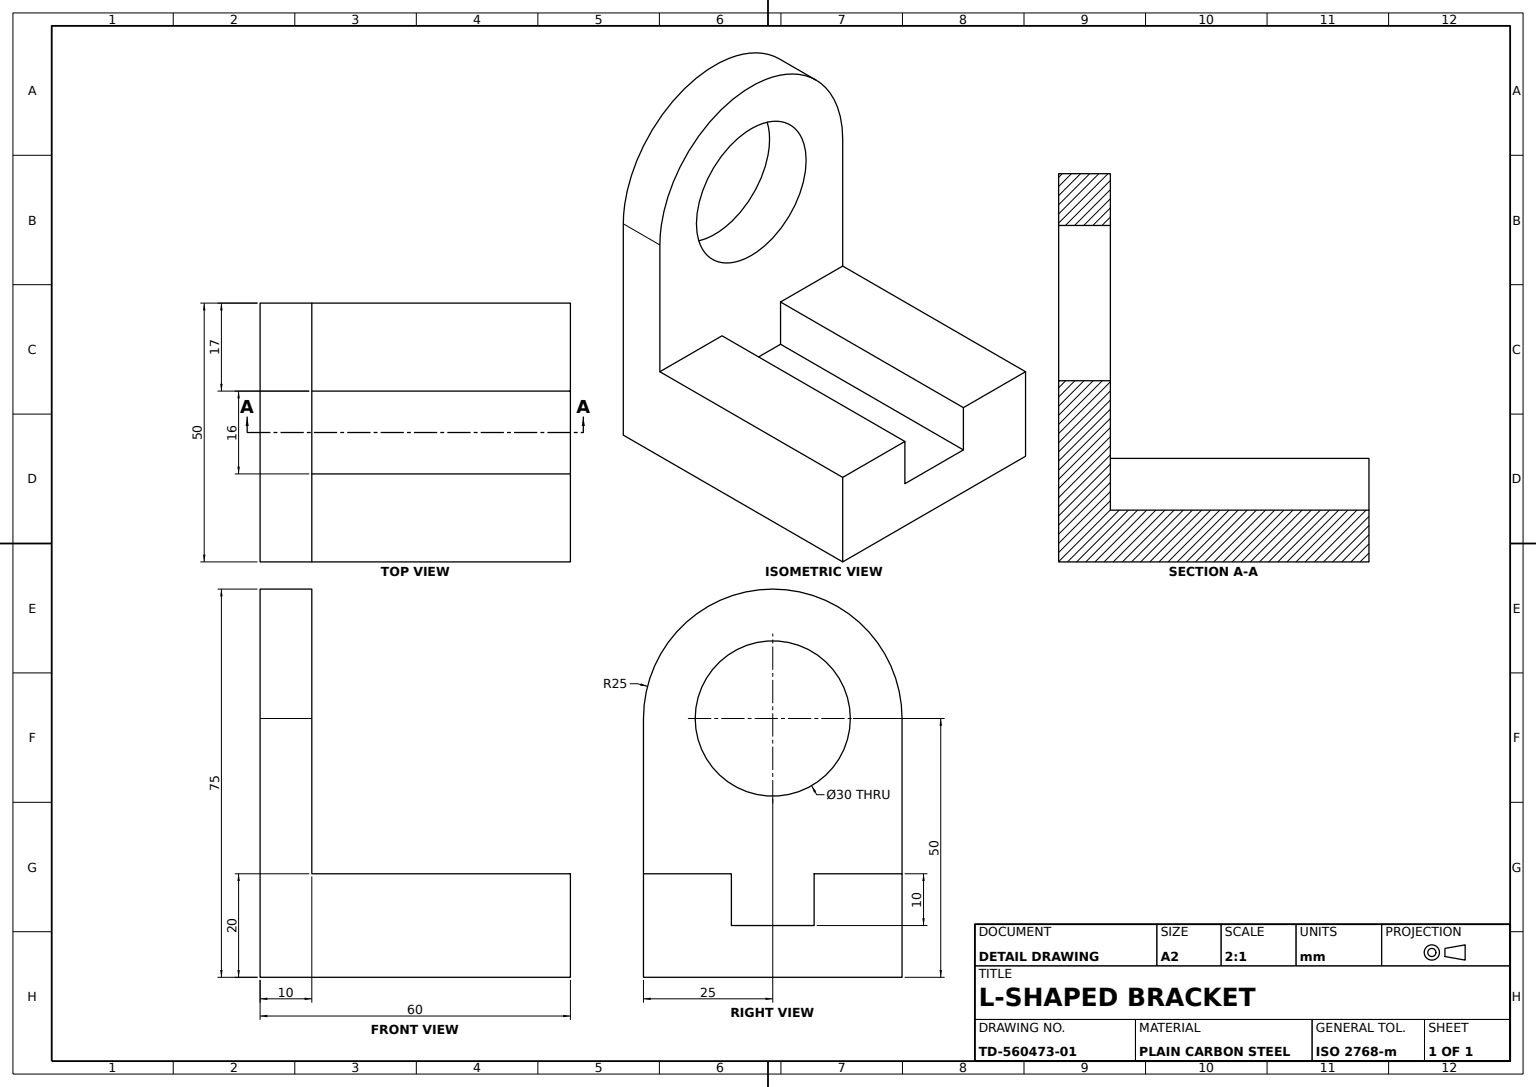
from build123d import *

# Parameters (mm, degrees)
BASE_BLOCK_SKETCH_W  = 60
BASE_BLOCK_SKETCH_H  = 50
BASE_BLOCK_DEPTH     = 20
UPRIGHT_SKETCH_W     = 10
UPRIGHT_SKETCH_H     = 50
UPRIGHT_DEPTH        = 30
ROUNDED_TOP_SKETCH_R = 25
ROUNDED_TOP_DEPTH    = 10
PIVOT_HOLE_SKETCH_R  = 15
PIVOT_HOLE_DEPTH     = 10
BASE_SLOT_SKETCH_W   = 16
BASE_SLOT_SKETCH_H   = 10
BASE_SLOT_DEPTH      = 50


with BuildPart() as part:
    # Base Block Sketch → Base Block (new body)
    with BuildSketch(Plane(origin=(0, 0, 0), x_dir=(1, 0, 0), z_dir=(0, 1, 0))):
        Rectangle(BASE_BLOCK_SKETCH_W, BASE_BLOCK_SKETCH_H)
    extrude(amount=BASE_BLOCK_DEPTH)

    # Upright Sketch → Upright (add)
    with BuildSketch(Plane(origin=(0, 20, 0), x_dir=(1, 0, 0), z_dir=(0, 1, 0))):
        with Locations((-25, 0)):
            Rectangle(UPRIGHT_SKETCH_W, UPRIGHT_SKETCH_H)
    extrude(amount=UPRIGHT_DEPTH)

    # Rounded Top Sketch → Rounded Top (add)
    with BuildSketch(Plane(origin=(-20, 0, 0), x_dir=(0, 0, -1), z_dir=(1, 0, 0))):
        with Locations((0, 50)):
            Circle(ROUNDED_TOP_SKETCH_R)
    extrude(amount=-ROUNDED_TOP_DEPTH)

    # Pivot Hole Sketch → Pivot Hole (cut)
    with BuildSketch(Plane(origin=(-20, 0, 0), x_dir=(0, 0, -1), z_dir=(1, 0, 0))):
        with Locations((0, 50)):
            Circle(PIVOT_HOLE_SKETCH_R)
    extrude(amount=-PIVOT_HOLE_DEPTH, mode=Mode.SUBTRACT)

    # Base Slot Sketch → Base Slot (cut)
    with BuildSketch(Plane(origin=(30, 0, 0), x_dir=(0, 0, -1), z_dir=(1, 0, 0))):
        with Locations((0, 15)):
            Rectangle(BASE_SLOT_SKETCH_W, BASE_SLOT_SKETCH_H)
    extrude(amount=-BASE_SLOT_DEPTH, mode=Mode.SUBTRACT)


solid = part.part
